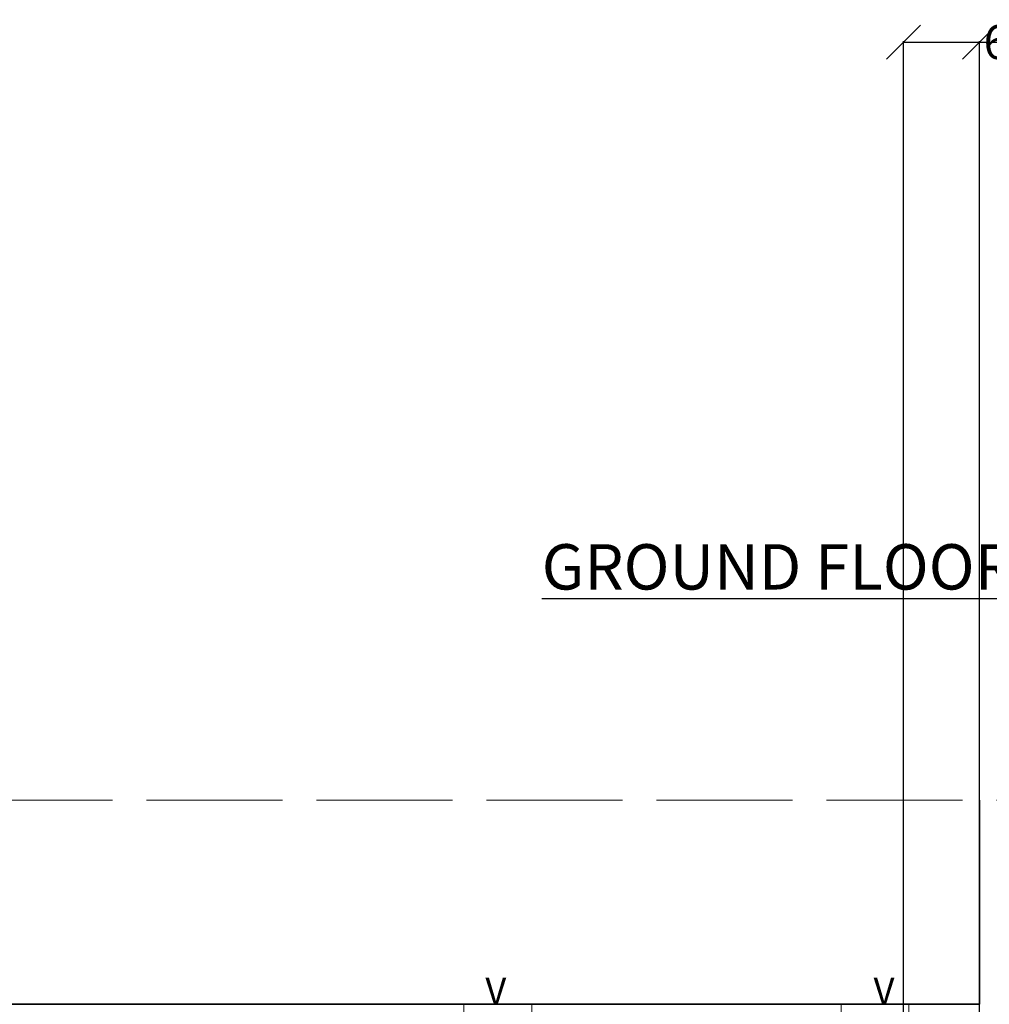
# Model space of a CAD drawing. Units: inches. Extents: x -1198 to -69, y -512 to 437.
# Tile 25 of 50: x -867 to -696, y 263 to 437. Entities that reach past the tile are written whole.
import ezdxf

# ---------------------------------------------------------------- set-up
doc = ezdxf.new("R2010")
doc.units = ezdxf.units.IN
doc.header["$MEASUREMENT"] = 0
doc.linetypes.add('ACAD_ISO02W100', pattern=[15, 12, -3])
for name, color, linetype, lineweight in [('A-ANNO-DIMS', 2, 'Continuous', 18), ('A-ANNO-SYMB', 7, 'Continuous', 18), ('A-ANNO-TEXT', 7, 'Continuous', 25), ('A-WALL', 7, 'Continuous', 35), ('C-PROP', 141, 'ACAD_ISO02W100', 18), ('windows', 160, 'Continuous', 18)]:
    doc.layers.add(name, color=color, linetype=linetype, lineweight=lineweight)
doc.styles.get("Standard").update_dxf_attribs({"font": 'arial.ttf'})
doc.dimstyles.get("Standard").update_dxf_attribs({"dimtxt": 6, "dimasz": 6, "dimexe": 0.18, "dimexo": 0.0625, "dimgap": 0.09, "dimtad": 0, "dimtih": 1, "dimtoh": 1, "dimdec": 0, "dimzin": 0, "dimdsep": 46, "dimlunit": 4, "dimtxsty": 'Standard', "dimblk": 'OBLIQUE', "dimcen": 0.09, "dimadec": 0, "dimazin": 0, "dimtfac": 1, "dimtdec": 0, "dimtofl": 0, "dimtmove": 0, "dimatfit": 3, "dimfxl": 1, "dimtolj": 1, "dimtzin": 0, "dimarcsym": 0})

# ---------------------------------------------------------------- blocks, each defined once
blk = doc.blocks.new('VENT-12')
at = {"ltscale": 10}
for p, q in [((0, 6), (0, 0)), ((12, 6), (12, 0)), ((0, 3), (12, 3))]:
    blk.add_line(p, q, dxfattribs=at)
blk = doc.blocks.new('_Oblique')
at = {"color": 0, "linetype": 'ByBlock', "lineweight": -2}
blk.add_line((-0.5, -0.5), (0.5, 0.5), dxfattribs=at)
blk = doc.blocks.new('*D73')
at = {"layer": 'A-ANNO-DIMS', "color": 0, "lineweight": -2, "ltscale": 10, "transparency": 16777216}
for p, q in [((-697.75, 299.29), (-697.75, 433.18)), ((-697.75, 433), (-696.82, 433)), ((-691.75, 433), (-692.68, 433)), ((-691.75, 299.29), (-691.75, 433.18))]:
    blk.add_line(p, q, dxfattribs=at)
at = {"layer": 'DEFPOINTS', "color": 0, "ltscale": 10, "transparency": 16777216}
for p in [(-691.75, 433), (-697.75, 299.23), (-691.75, 299.23)]:
    blk.add_point(p, dxfattribs=at)
at = {"layer": 'A-ANNO-DIMS', "color": 0, "lineweight": -2, "ltscale": 10, "transparency": 16777216, "xscale": 6, "yscale": 6, "zscale": 6, "rotation": 180}
blk.add_blockref('_Oblique', (-697.75, 433), dxfattribs=at)
at = {"layer": 'A-ANNO-DIMS', "color": 0, "lineweight": -2, "ltscale": 10, "transparency": 16777216, "xscale": 6, "yscale": 6, "zscale": 6}
blk.add_blockref('_Oblique', (-691.75, 433), dxfattribs=at)
at = {"layer": 'A-ANNO-DIMS', "color": 0, "ltscale": 10, "transparency": 16777216, "insert": (-694.75, 433), "char_height": 6, "attachment_point": 5}
blk.add_mtext('\\A1;6', dxfattribs=at)
blk = doc.blocks.new('*D76')
at = {"layer": 'A-ANNO-DIMS', "color": 0, "lineweight": -2, "ltscale": 10, "transparency": 16777216}
for p, q in [((-711.13, -38.21), (-711.13, 433.18)), ((-711.13, 433), (-697.75, 433)), ((-697.75, -38.21), (-697.75, 433.18)), ((-697.75, 433), (-691.75, 433))]:
    blk.add_line(p, q, dxfattribs=at)
at = {"layer": 'DEFPOINTS', "color": 0, "ltscale": 10, "transparency": 16777216}
for p in [(-697.75, 433), (-711.13, -38.27), (-697.75, -38.27)]:
    blk.add_point(p, dxfattribs=at)
at = {"layer": 'A-ANNO-DIMS', "color": 0, "lineweight": -2, "ltscale": 10, "transparency": 16777216, "xscale": 6, "yscale": 6, "zscale": 6, "rotation": 180}
blk.add_blockref('_Oblique', (-711.13, 433), dxfattribs=at)
at = {"layer": 'A-ANNO-DIMS', "color": 0, "lineweight": -2, "ltscale": 10, "transparency": 16777216, "xscale": 6, "yscale": 6, "zscale": 6}
blk.add_blockref('_Oblique', (-697.75, 433), dxfattribs=at)
at = {"layer": 'A-ANNO-DIMS', "color": 0, "ltscale": 10, "transparency": 16777216, "insert": (-681.81, 433), "char_height": 6, "attachment_point": 5}
blk.add_mtext('\\A1;13.38', dxfattribs=at)

msp = doc.modelspace()

# ---------------------------------------------------------------- linework, layer by layer
at = {"layer": 'A-WALL', "ltscale": 10}
for p, q in [((-697.7509, 299.2277), (-697.7509, 263.2277)), ((-697.7509, 263.2277), (-1018.7509, 263.2277))]:
    msp.add_line(p, q, dxfattribs=at)
at = {"layer": 'C-PROP', "ltscale": 2}
msp.add_lwpolyline([(-1054.7509, 299.2277), (-334.7509, 299.2277), (-334.7509, -264.7723), (-1054.7509, -264.7723)], close=True, dxfattribs=at)

# ---------------------------------------------------------------- block references
at = {"layer": 'windows', "rotation": 180}
msp.add_blockref('VENT-12', (-776.7361, 263.2273), dxfattribs=at)
at = {"layer": 'windows'}
msp.add_blockref('VENT-12', (-722.179, 257.228), dxfattribs=at)

# ---------------------------------------------------------------- texts
at = {"layer": 'A-ANNO-SYMB', "ltscale": 10}
for p in [(-784.9547, 263.2277), (-716.4315, 263.2277)]:
    msp.add_text('V', height=4.6996, dxfattribs=at).set_placement(p)
at = {"layer": 'A-ANNO-TEXT', "ltscale": 10, "insert": (-775.0037, 344.4033), "char_height": 8, "attachment_point": 1}
msp.add_mtext_dynamic_manual_height_columns('{\\fArial|b1|i0|c0|p34;\\LGROUND FLOOR PLAN}', width=340.81761, gutter_width=40, heights=[0], dxfattribs=at)

# ---------------------------------------------------------------- dimensions: what is measured, and where the dimension line sits
at = {"layer": 'A-ANNO-DIMS', "ltscale": 10}
for base, p1, p2, override, picture, middle in [((-697.7509, 433.0036), (-711.1319, -38.2723), (-697.7509, -38.2723), {"dimdec": 2, "dimlfac": 1, "dimrnd": 0, "dimzin": 0, "dimdsep": 46, "dimlunit": 2}, '*D76', (-681.8137, 433.0036)), ((-691.7509, 433.0036), (-697.7509, 299.2277), (-691.7509, 299.2277), {"dimdec": 0, "dimlfac": 1, "dimrnd": 0, "dimzin": 0, "dimdsep": 46, "dimlunit": 2}, '*D73', (-694.7509, 433.0036))]:
    dim = msp.add_linear_dim(base=base, p1=p1, p2=p2, dimstyle='Standard', override=override, dxfattribs=at)
    dim.commit()
    dim.dimension.update_dxf_attribs({"geometry": picture, "text_midpoint": middle})

doc.saveas('drawing.dxf')
